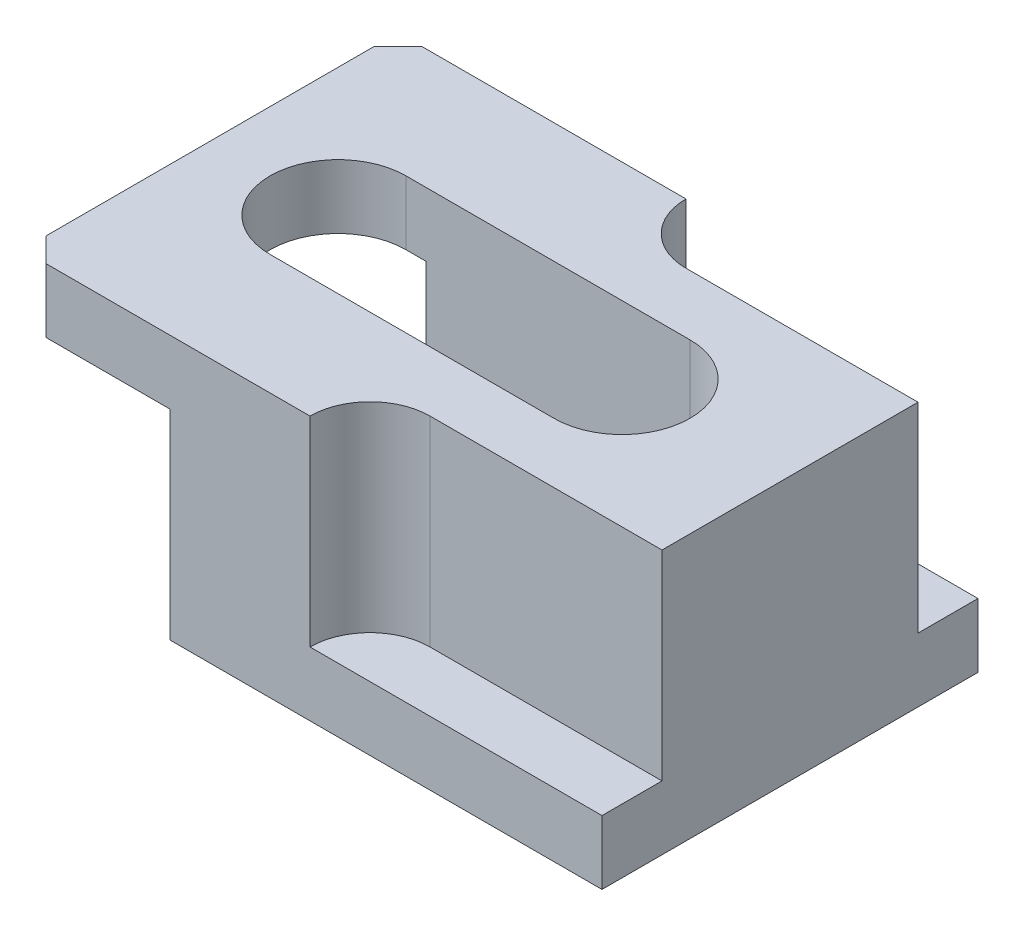
ISO-10303-21;
HEADER;
FILE_DESCRIPTION(('STEP AP214'),'2;1');
FILE_NAME('part.step','',(''),(''),'','','');
FILE_SCHEMA(('AUTOMOTIVE_DESIGN { 1 0 10303 214 1 1 1 1 }'));
ENDSEC;
DATA;
#1=APPLICATION_CONTEXT('core data for automotive mechanical design processes');
#2=APPLICATION_PROTOCOL_DEFINITION('international standard','automotive_design',2000,#1);
#3=PRODUCT_CONTEXT('',#1,'mechanical');
#4=PRODUCT('Part','Part','',(#3));
#5=PRODUCT_RELATED_PRODUCT_CATEGORY('part','',(#4));
#6=PRODUCT_DEFINITION_FORMATION('','',#4);
#7=PRODUCT_DEFINITION_CONTEXT('part definition',#1,'design');
#8=PRODUCT_DEFINITION('design','',#6,#7);
#9=PRODUCT_DEFINITION_SHAPE('','',#8);
#10=(LENGTH_UNIT() NAMED_UNIT(*) SI_UNIT(.MILLI.,.METRE.));
#11=(NAMED_UNIT(*) PLANE_ANGLE_UNIT() SI_UNIT($,.RADIAN.));
#12=(NAMED_UNIT(*) SI_UNIT($,.STERADIAN.) SOLID_ANGLE_UNIT());
#13=UNCERTAINTY_MEASURE_WITH_UNIT(LENGTH_MEASURE(1.E-05),#10,'distance_accuracy_value','');
#14=(GEOMETRIC_REPRESENTATION_CONTEXT(3) GLOBAL_UNCERTAINTY_ASSIGNED_CONTEXT((#13)) GLOBAL_UNIT_ASSIGNED_CONTEXT((#10,
#11,#12)) REPRESENTATION_CONTEXT('',''));
#15=CARTESIAN_POINT('',(0.,0.,0.));
#16=DIRECTION('',(0.,0.,1.));
#17=DIRECTION('',(1.,0.,0.));
#18=AXIS2_PLACEMENT_3D('',#15,#16,#17);
#19=CARTESIAN_POINT('',(0.,25.,-47.));
#20=DIRECTION('',(-1.,0.,0.));
#21=DIRECTION('',(0.,-1.,0.));
#22=AXIS2_PLACEMENT_3D('',#19,#20,#21);
#23=PLANE('',#22);
#24=DIRECTION('',(0.,-1.,0.));
#25=VECTOR('',#24,1.);
#26=CARTESIAN_POINT('',(0.,25.,-32.));
#27=LINE('',#26,#25);
#28=CARTESIAN_POINT('',(0.,25.,-32.));
#29=VERTEX_POINT('',#28);
#30=CARTESIAN_POINT('',(0.,8.,-32.));
#31=VERTEX_POINT('',#30);
#32=EDGE_CURVE('E237',#29,#31,#27,.T.);
#33=ORIENTED_EDGE('',*,*,#32,.F.);
#34=DIRECTION('',(0.,0.,1.));
#35=VECTOR('',#34,1.);
#36=CARTESIAN_POINT('',(0.,25.,-47.));
#37=LINE('',#36,#35);
#38=CARTESIAN_POINT('',(0.,25.,-47.));
#39=VERTEX_POINT('',#38);
#40=EDGE_CURVE('E315',#39,#29,#37,.T.);
#41=ORIENTED_EDGE('',*,*,#40,.F.);
#42=DIRECTION('',(0.,-1.,0.));
#43=VECTOR('',#42,1.);
#44=CARTESIAN_POINT('',(0.,25.,-47.));
#45=LINE('',#44,#43);
#46=CARTESIAN_POINT('',(0.,0.,-47.));
#47=VERTEX_POINT('',#46);
#48=EDGE_CURVE('E289',#39,#47,#45,.T.);
#49=ORIENTED_EDGE('',*,*,#48,.T.);
#50=DIRECTION('',(0.,0.,1.));
#51=VECTOR('',#50,1.);
#52=CARTESIAN_POINT('',(0.,0.,-47.));
#53=LINE('',#52,#51);
#54=CARTESIAN_POINT('',(0.,0.,0.));
#55=VERTEX_POINT('',#54);
#56=EDGE_CURVE('E300',#47,#55,#53,.T.);
#57=ORIENTED_EDGE('',*,*,#56,.T.);
#58=DIRECTION('',(0.,-1.,0.));
#59=VECTOR('',#58,1.);
#60=CARTESIAN_POINT('',(0.,25.,0.));
#61=LINE('',#60,#59);
#62=CARTESIAN_POINT('',(0.,25.,0.));
#63=VERTEX_POINT('',#62);
#64=EDGE_CURVE('E281',#63,#55,#61,.T.);
#65=ORIENTED_EDGE('',*,*,#64,.F.);
#66=CARTESIAN_POINT('',(0.,25.,-15.));
#67=VERTEX_POINT('',#66);
#68=EDGE_CURVE('E312',#67,#63,#37,.T.);
#69=ORIENTED_EDGE('',*,*,#68,.F.);
#70=DIRECTION('',(0.,1.,0.));
#71=VECTOR('',#70,1.);
#72=CARTESIAN_POINT('',(0.,25.,-15.));
#73=LINE('',#72,#71);
#74=CARTESIAN_POINT('',(0.,8.,-15.));
#75=VERTEX_POINT('',#74);
#76=EDGE_CURVE('E231',#75,#67,#73,.T.);
#77=ORIENTED_EDGE('',*,*,#76,.F.);
#78=DIRECTION('',(0.,0.,-1.));
#79=VECTOR('',#78,1.);
#80=CARTESIAN_POINT('',(0.,8.,-47.));
#81=LINE('',#80,#79);
#82=EDGE_CURVE('E197',#75,#31,#81,.T.);
#83=ORIENTED_EDGE('',*,*,#82,.T.);
#84=EDGE_LOOP('',(#33,#41,#49,#57,#65,#69,#77,#83));
#85=FACE_BOUND('',#84,.T.);
#86=ADVANCED_FACE('F50',(#85),#23,.T.);
#87=CARTESIAN_POINT('',(-18.5,25.,-47.));
#88=DIRECTION('',(0.,-1.,0.));
#89=DIRECTION('',(0.,0.,-1.));
#90=AXIS2_PLACEMENT_3D('',#87,#88,#89);
#91=PLANE('',#90);
#92=DIRECTION('',(0.,0.,1.));
#93=VECTOR('',#92,1.);
#94=CARTESIAN_POINT('',(-18.5,25.,-47.));
#95=LINE('',#94,#93);
#96=CARTESIAN_POINT('',(-18.5,25.,-44.));
#97=VERTEX_POINT('',#96);
#98=CARTESIAN_POINT('',(-18.5,25.,-3.));
#99=VERTEX_POINT('',#98);
#100=EDGE_CURVE('E316',#97,#99,#95,.T.);
#101=ORIENTED_EDGE('',*,*,#100,.F.);
#102=DIRECTION('',(0.707106781186549,0.,-0.707106781186546));
#103=VECTOR('',#102,1.);
#104=CARTESIAN_POINT('',(-17.,25.,-45.5));
#105=LINE('',#104,#103);
#106=CARTESIAN_POINT('',(-15.5,25.,-47.));
#107=VERTEX_POINT('',#106);
#108=EDGE_CURVE('E333',#97,#107,#105,.T.);
#109=ORIENTED_EDGE('',*,*,#108,.T.);
#110=DIRECTION('',(1.,0.,0.));
#111=VECTOR('',#110,1.);
#112=CARTESIAN_POINT('',(-18.5,25.,-47.));
#113=LINE('',#112,#111);
#114=EDGE_CURVE('E299',#107,#39,#113,.T.);
#115=ORIENTED_EDGE('',*,*,#114,.T.);
#116=ORIENTED_EDGE('',*,*,#40,.T.);
#117=DIRECTION('',(1.,0.,0.));
#118=VECTOR('',#117,1.);
#119=CARTESIAN_POINT('',(-18.5,25.,-32.));
#120=LINE('',#119,#118);
#121=CARTESIAN_POINT('',(-2.5,25.,-32.));
#122=VERTEX_POINT('',#121);
#123=EDGE_CURVE('E233',#122,#29,#120,.T.);
#124=ORIENTED_EDGE('',*,*,#123,.F.);
#125=CARTESIAN_POINT('',(-2.5,25.,-23.5));
#126=DIRECTION('',(0.,-1.,0.));
#127=DIRECTION('',(0.,0.,-1.));
#128=AXIS2_PLACEMENT_3D('',#125,#126,#127);
#129=CIRCLE('',#128,8.5);
#130=CARTESIAN_POINT('',(-2.5,25.,-15.));
#131=VERTEX_POINT('',#130);
#132=EDGE_CURVE('E236',#131,#122,#129,.T.);
#133=ORIENTED_EDGE('',*,*,#132,.F.);
#134=DIRECTION('',(-1.,0.,0.));
#135=VECTOR('',#134,1.);
#136=CARTESIAN_POINT('',(-18.5,25.,-15.));
#137=LINE('',#136,#135);
#138=EDGE_CURVE('E229',#67,#131,#137,.T.);
#139=ORIENTED_EDGE('',*,*,#138,.F.);
#140=ORIENTED_EDGE('',*,*,#68,.T.);
#141=DIRECTION('',(1.,0.,0.));
#142=VECTOR('',#141,1.);
#143=CARTESIAN_POINT('',(-18.5,25.,0.));
#144=LINE('',#143,#142);
#145=CARTESIAN_POINT('',(-15.5,25.,0.));
#146=VERTEX_POINT('',#145);
#147=EDGE_CURVE('E287',#146,#63,#144,.T.);
#148=ORIENTED_EDGE('',*,*,#147,.F.);
#149=DIRECTION('',(0.707106781186548,0.,0.707106781186548));
#150=VECTOR('',#149,1.);
#151=CARTESIAN_POINT('',(-40.5,25.,-25.));
#152=LINE('',#151,#150);
#153=EDGE_CURVE('E334',#146,#99,#152,.F.);
#154=ORIENTED_EDGE('',*,*,#153,.T.);
#155=EDGE_LOOP('',(#101,#109,#115,#116,#124,#133,#139,#140,#148,#154));
#156=FACE_BOUND('',#155,.T.);
#157=ADVANCED_FACE('F348',(#156),#91,.T.);
#158=CARTESIAN_POINT('',(-18.5,33.,-47.));
#159=DIRECTION('',(-1.,0.,0.));
#160=DIRECTION('',(0.,0.,1.));
#161=AXIS2_PLACEMENT_3D('',#158,#159,#160);
#162=PLANE('',#161);
#163=DIRECTION('',(0.,0.,1.));
#164=VECTOR('',#163,1.);
#165=CARTESIAN_POINT('',(-18.5,33.,-47.));
#166=LINE('',#165,#164);
#167=CARTESIAN_POINT('',(-18.5,33.,-44.));
#168=VERTEX_POINT('',#167);
#169=CARTESIAN_POINT('',(-18.5,33.,-3.));
#170=VERTEX_POINT('',#169);
#171=EDGE_CURVE('E317',#168,#170,#166,.T.);
#172=ORIENTED_EDGE('',*,*,#171,.F.);
#173=DIRECTION('',(0.,-1.,0.));
#174=VECTOR('',#173,1.);
#175=CARTESIAN_POINT('',(-18.5,25.,-44.));
#176=LINE('',#175,#174);
#177=EDGE_CURVE('E329',#168,#97,#176,.T.);
#178=ORIENTED_EDGE('',*,*,#177,.T.);
#179=ORIENTED_EDGE('',*,*,#100,.T.);
#180=DIRECTION('',(0.,1.,0.));
#181=VECTOR('',#180,1.);
#182=CARTESIAN_POINT('',(-18.5,33.,-3.));
#183=LINE('',#182,#181);
#184=EDGE_CURVE('E327',#99,#170,#183,.T.);
#185=ORIENTED_EDGE('',*,*,#184,.T.);
#186=EDGE_LOOP('',(#172,#178,#179,#185));
#187=FACE_BOUND('',#186,.T.);
#188=ADVANCED_FACE('F342',(#187),#162,.T.);
#189=CARTESIAN_POINT('',(54.,33.,-47.));
#190=DIRECTION('',(0.,1.,0.));
#191=DIRECTION('',(0.,0.,1.));
#192=AXIS2_PLACEMENT_3D('',#189,#190,#191);
#193=PLANE('',#192);
#194=CARTESIAN_POINT('',(-2.5,33.,-23.5));
#195=DIRECTION('',(0.,1.,0.));
#196=DIRECTION('',(0.,0.,1.));
#197=AXIS2_PLACEMENT_3D('',#194,#195,#196);
#198=CIRCLE('',#197,8.5);
#199=CARTESIAN_POINT('',(-2.5,33.,-32.));
#200=VERTEX_POINT('',#199);
#201=CARTESIAN_POINT('',(-2.5,33.,-15.));
#202=VERTEX_POINT('',#201);
#203=EDGE_CURVE('E218',#200,#202,#198,.T.);
#204=ORIENTED_EDGE('',*,*,#203,.F.);
#205=DIRECTION('',(-1.,0.,0.));
#206=VECTOR('',#205,1.);
#207=CARTESIAN_POINT('',(-2.5,33.,-32.));
#208=LINE('',#207,#206);
#209=CARTESIAN_POINT('',(33.,33.,-32.));
#210=VERTEX_POINT('',#209);
#211=EDGE_CURVE('E199',#210,#200,#208,.T.);
#212=ORIENTED_EDGE('',*,*,#211,.F.);
#213=CARTESIAN_POINT('',(33.,33.,-23.5));
#214=DIRECTION('',(0.,1.,0.));
#215=DIRECTION('',(0.,0.,1.));
#216=AXIS2_PLACEMENT_3D('',#213,#214,#215);
#217=CIRCLE('',#216,8.5);
#218=CARTESIAN_POINT('',(33.,33.,-15.));
#219=VERTEX_POINT('',#218);
#220=EDGE_CURVE('E225',#219,#210,#217,.T.);
#221=ORIENTED_EDGE('',*,*,#220,.F.);
#222=DIRECTION('',(1.,0.,0.));
#223=VECTOR('',#222,1.);
#224=CARTESIAN_POINT('',(-2.5,33.,-15.));
#225=LINE('',#224,#223);
#226=EDGE_CURVE('E210',#202,#219,#225,.T.);
#227=ORIENTED_EDGE('',*,*,#226,.F.);
#228=EDGE_LOOP('',(#204,#212,#221,#227));
#229=FACE_BOUND('',#228,.T.);
#230=DIRECTION('',(-1.,0.,0.));
#231=VECTOR('',#230,1.);
#232=CARTESIAN_POINT('',(54.,33.,-47.));
#233=LINE('',#232,#231);
#234=CARTESIAN_POINT('',(17.5,33.,-47.));
#235=VERTEX_POINT('',#234);
#236=CARTESIAN_POINT('',(-15.5,33.,-47.));
#237=VERTEX_POINT('',#236);
#238=EDGE_CURVE('E296',#235,#237,#233,.T.);
#239=ORIENTED_EDGE('',*,*,#238,.T.);
#240=DIRECTION('',(-0.707106781186549,0.,0.707106781186546));
#241=VECTOR('',#240,1.);
#242=CARTESIAN_POINT('',(19.2500000000002,33.,-81.75));
#243=LINE('',#242,#241);
#244=EDGE_CURVE('E57',#237,#168,#243,.T.);
#245=ORIENTED_EDGE('',*,*,#244,.T.);
#246=ORIENTED_EDGE('',*,*,#171,.T.);
#247=DIRECTION('',(-0.707106781186548,0.,-0.707106781186548));
#248=VECTOR('',#247,1.);
#249=CARTESIAN_POINT('',(-4.25,33.,11.25));
#250=LINE('',#249,#248);
#251=CARTESIAN_POINT('',(-15.5,33.,0.));
#252=VERTEX_POINT('',#251);
#253=EDGE_CURVE('E64',#170,#252,#250,.F.);
#254=ORIENTED_EDGE('',*,*,#253,.T.);
#255=DIRECTION('',(-1.,0.,0.));
#256=VECTOR('',#255,1.);
#257=CARTESIAN_POINT('',(54.,33.,0.));
#258=LINE('',#257,#256);
#259=CARTESIAN_POINT('',(17.5,33.,0.));
#260=VERTEX_POINT('',#259);
#261=EDGE_CURVE('E310',#260,#252,#258,.T.);
#262=ORIENTED_EDGE('',*,*,#261,.F.);
#263=CARTESIAN_POINT('',(25.,33.,0.));
#264=DIRECTION('',(0.,1.,0.));
#265=DIRECTION('',(0.,0.,1.));
#266=AXIS2_PLACEMENT_3D('',#263,#264,#265);
#267=CIRCLE('',#266,7.5);
#268=CARTESIAN_POINT('',(25.,33.,-7.5));
#269=VERTEX_POINT('',#268);
#270=EDGE_CURVE('E266',#269,#260,#267,.T.);
#271=ORIENTED_EDGE('',*,*,#270,.F.);
#272=DIRECTION('',(-1.,0.,0.));
#273=VECTOR('',#272,1.);
#274=CARTESIAN_POINT('',(54.,33.,-7.5));
#275=LINE('',#274,#273);
#276=CARTESIAN_POINT('',(54.,33.,-7.5));
#277=VERTEX_POINT('',#276);
#278=EDGE_CURVE('E259',#277,#269,#275,.T.);
#279=ORIENTED_EDGE('',*,*,#278,.F.);
#280=DIRECTION('',(0.,0.,1.));
#281=VECTOR('',#280,1.);
#282=CARTESIAN_POINT('',(54.,33.,-47.));
#283=LINE('',#282,#281);
#284=CARTESIAN_POINT('',(54.,33.,-39.5));
#285=VERTEX_POINT('',#284);
#286=EDGE_CURVE('E321',#285,#277,#283,.T.);
#287=ORIENTED_EDGE('',*,*,#286,.F.);
#288=DIRECTION('',(1.,0.,0.));
#289=VECTOR('',#288,1.);
#290=CARTESIAN_POINT('',(54.,33.,-39.5));
#291=LINE('',#290,#289);
#292=CARTESIAN_POINT('',(25.,33.,-39.5));
#293=VERTEX_POINT('',#292);
#294=EDGE_CURVE('E243',#293,#285,#291,.T.);
#295=ORIENTED_EDGE('',*,*,#294,.F.);
#296=CARTESIAN_POINT('',(25.,33.,-47.));
#297=DIRECTION('',(0.,1.,0.));
#298=DIRECTION('',(0.,0.,1.));
#299=AXIS2_PLACEMENT_3D('',#296,#297,#298);
#300=CIRCLE('',#299,7.5);
#301=EDGE_CURVE('E238',#235,#293,#300,.T.);
#302=ORIENTED_EDGE('',*,*,#301,.F.);
#303=EDGE_LOOP('',(#239,#245,#246,#254,#262,#271,#279,#287,#295,#302));
#304=FACE_BOUND('',#303,.T.);
#305=ADVANCED_FACE('F340',(#229,#304),#193,.T.);
#306=CARTESIAN_POINT('',(54.,8.,-47.));
#307=DIRECTION('',(1.,0.,0.));
#308=DIRECTION('',(0.,0.,-1.));
#309=AXIS2_PLACEMENT_3D('',#306,#307,#308);
#310=PLANE('',#309);
#311=DIRECTION('',(0.,1.,0.));
#312=VECTOR('',#311,1.);
#313=CARTESIAN_POINT('',(54.,8.,-39.5));
#314=LINE('',#313,#312);
#315=CARTESIAN_POINT('',(54.,8.,-39.5));
#316=VERTEX_POINT('',#315);
#317=EDGE_CURVE('E258',#316,#285,#314,.T.);
#318=ORIENTED_EDGE('',*,*,#317,.T.);
#319=ORIENTED_EDGE('',*,*,#286,.T.);
#320=DIRECTION('',(0.,1.,0.));
#321=VECTOR('',#320,1.);
#322=CARTESIAN_POINT('',(54.,8.,-7.5));
#323=LINE('',#322,#321);
#324=CARTESIAN_POINT('',(54.,8.,-7.5));
#325=VERTEX_POINT('',#324);
#326=EDGE_CURVE('E273',#325,#277,#323,.T.);
#327=ORIENTED_EDGE('',*,*,#326,.F.);
#328=DIRECTION('',(0.,0.,-1.));
#329=VECTOR('',#328,1.);
#330=CARTESIAN_POINT('',(54.,8.,0.));
#331=LINE('',#330,#329);
#332=CARTESIAN_POINT('',(54.,8.,0.));
#333=VERTEX_POINT('',#332);
#334=EDGE_CURVE('E264',#333,#325,#331,.T.);
#335=ORIENTED_EDGE('',*,*,#334,.F.);
#336=DIRECTION('',(0.,1.,0.));
#337=VECTOR('',#336,1.);
#338=CARTESIAN_POINT('',(54.,8.,0.));
#339=LINE('',#338,#337);
#340=CARTESIAN_POINT('',(54.,0.,0.));
#341=VERTEX_POINT('',#340);
#342=EDGE_CURVE('E308',#341,#333,#339,.T.);
#343=ORIENTED_EDGE('',*,*,#342,.F.);
#344=DIRECTION('',(0.,0.,1.));
#345=VECTOR('',#344,1.);
#346=CARTESIAN_POINT('',(54.,0.,-47.));
#347=LINE('',#346,#345);
#348=CARTESIAN_POINT('',(54.,0.,-47.));
#349=VERTEX_POINT('',#348);
#350=EDGE_CURVE('E323',#349,#341,#347,.T.);
#351=ORIENTED_EDGE('',*,*,#350,.F.);
#352=DIRECTION('',(0.,1.,0.));
#353=VECTOR('',#352,1.);
#354=CARTESIAN_POINT('',(54.,0.,-47.));
#355=LINE('',#354,#353);
#356=CARTESIAN_POINT('',(54.,8.,-47.));
#357=VERTEX_POINT('',#356);
#358=EDGE_CURVE('E291',#349,#357,#355,.T.);
#359=ORIENTED_EDGE('',*,*,#358,.T.);
#360=DIRECTION('',(0.,0.,-1.));
#361=VECTOR('',#360,1.);
#362=CARTESIAN_POINT('',(54.,8.,-47.));
#363=LINE('',#362,#361);
#364=EDGE_CURVE('E247',#316,#357,#363,.T.);
#365=ORIENTED_EDGE('',*,*,#364,.F.);
#366=EDGE_LOOP('',(#318,#319,#327,#335,#343,#351,#359,#365));
#367=FACE_BOUND('',#366,.T.);
#368=ADVANCED_FACE('F373',(#367),#310,.T.);
#369=CARTESIAN_POINT('',(0.,0.,-47.));
#370=DIRECTION('',(0.,-1.,0.));
#371=DIRECTION('',(0.,0.,-1.));
#372=AXIS2_PLACEMENT_3D('',#369,#370,#371);
#373=PLANE('',#372);
#374=DIRECTION('',(1.,0.,0.));
#375=VECTOR('',#374,1.);
#376=CARTESIAN_POINT('',(0.,0.,0.));
#377=LINE('',#376,#375);
#378=EDGE_CURVE('E305',#55,#341,#377,.T.);
#379=ORIENTED_EDGE('',*,*,#378,.F.);
#380=ORIENTED_EDGE('',*,*,#56,.F.);
#381=DIRECTION('',(1.,0.,0.));
#382=VECTOR('',#381,1.);
#383=CARTESIAN_POINT('',(0.,0.,-47.));
#384=LINE('',#383,#382);
#385=EDGE_CURVE('E288',#47,#349,#384,.T.);
#386=ORIENTED_EDGE('',*,*,#385,.T.);
#387=ORIENTED_EDGE('',*,*,#350,.T.);
#388=EDGE_LOOP('',(#379,#380,#386,#387));
#389=FACE_BOUND('',#388,.T.);
#390=ADVANCED_FACE('F379',(#389),#373,.T.);
#391=CARTESIAN_POINT('',(0.,0.,-47.));
#392=DIRECTION('',(0.,0.,1.));
#393=DIRECTION('',(1.,0.,0.));
#394=AXIS2_PLACEMENT_3D('',#391,#392,#393);
#395=PLANE('',#394);
#396=ORIENTED_EDGE('',*,*,#114,.F.);
#397=DIRECTION('',(0.,1.,0.));
#398=VECTOR('',#397,1.);
#399=CARTESIAN_POINT('',(-15.5,33.,-47.));
#400=LINE('',#399,#398);
#401=EDGE_CURVE('E72',#107,#237,#400,.T.);
#402=ORIENTED_EDGE('',*,*,#401,.T.);
#403=ORIENTED_EDGE('',*,*,#238,.F.);
#404=DIRECTION('',(0.,1.,0.));
#405=VECTOR('',#404,1.);
#406=CARTESIAN_POINT('',(17.5,8.,-47.));
#407=LINE('',#406,#405);
#408=CARTESIAN_POINT('',(17.5,8.,-47.));
#409=VERTEX_POINT('',#408);
#410=EDGE_CURVE('E252',#409,#235,#407,.T.);
#411=ORIENTED_EDGE('',*,*,#410,.F.);
#412=DIRECTION('',(-1.,0.,0.));
#413=VECTOR('',#412,1.);
#414=CARTESIAN_POINT('',(25.,8.,-47.));
#415=LINE('',#414,#413);
#416=EDGE_CURVE('E241',#357,#409,#415,.T.);
#417=ORIENTED_EDGE('',*,*,#416,.F.);
#418=ORIENTED_EDGE('',*,*,#358,.F.);
#419=ORIENTED_EDGE('',*,*,#385,.F.);
#420=ORIENTED_EDGE('',*,*,#48,.F.);
#421=EDGE_LOOP('',(#396,#402,#403,#411,#417,#418,#419,#420));
#422=FACE_BOUND('',#421,.T.);
#423=ADVANCED_FACE('F354',(#422),#395,.F.);
#424=CARTESIAN_POINT('',(0.,0.,0.));
#425=DIRECTION('',(0.,0.,1.));
#426=DIRECTION('',(1.,0.,0.));
#427=AXIS2_PLACEMENT_3D('',#424,#425,#426);
#428=PLANE('',#427);
#429=ORIENTED_EDGE('',*,*,#261,.T.);
#430=DIRECTION('',(0.,-1.,0.));
#431=VECTOR('',#430,1.);
#432=CARTESIAN_POINT('',(-15.5,0.,0.));
#433=LINE('',#432,#431);
#434=EDGE_CURVE('E11',#252,#146,#433,.T.);
#435=ORIENTED_EDGE('',*,*,#434,.T.);
#436=ORIENTED_EDGE('',*,*,#147,.T.);
#437=ORIENTED_EDGE('',*,*,#64,.T.);
#438=ORIENTED_EDGE('',*,*,#378,.T.);
#439=ORIENTED_EDGE('',*,*,#342,.T.);
#440=DIRECTION('',(1.,0.,0.));
#441=VECTOR('',#440,1.);
#442=CARTESIAN_POINT('',(25.,8.,0.));
#443=LINE('',#442,#441);
#444=CARTESIAN_POINT('',(17.5,8.,0.));
#445=VERTEX_POINT('',#444);
#446=EDGE_CURVE('E263',#445,#333,#443,.T.);
#447=ORIENTED_EDGE('',*,*,#446,.F.);
#448=DIRECTION('',(0.,1.,0.));
#449=VECTOR('',#448,1.);
#450=CARTESIAN_POINT('',(17.5,8.,0.));
#451=LINE('',#450,#449);
#452=EDGE_CURVE('E279',#445,#260,#451,.T.);
#453=ORIENTED_EDGE('',*,*,#452,.T.);
#454=EDGE_LOOP('',(#429,#435,#436,#437,#438,#439,#447,#453));
#455=FACE_BOUND('',#454,.T.);
#456=ADVANCED_FACE('F432',(#455),#428,.T.);
#457=CARTESIAN_POINT('',(25.,8.,0.));
#458=DIRECTION('',(0.,1.,0.));
#459=DIRECTION('',(0.,0.,1.));
#460=AXIS2_PLACEMENT_3D('',#457,#458,#459);
#461=CYLINDRICAL_SURFACE('',#460,7.5);
#462=ORIENTED_EDGE('',*,*,#270,.T.);
#463=ORIENTED_EDGE('',*,*,#452,.F.);
#464=CARTESIAN_POINT('',(25.,8.,0.));
#465=DIRECTION('',(0.,1.,0.));
#466=DIRECTION('',(0.,0.,1.));
#467=AXIS2_PLACEMENT_3D('',#464,#465,#466);
#468=CIRCLE('',#467,7.5);
#469=CARTESIAN_POINT('',(25.,8.,-7.5));
#470=VERTEX_POINT('',#469);
#471=EDGE_CURVE('E275',#470,#445,#468,.T.);
#472=ORIENTED_EDGE('',*,*,#471,.F.);
#473=DIRECTION('',(0.,1.,0.));
#474=VECTOR('',#473,1.);
#475=CARTESIAN_POINT('',(25.,8.,-7.5));
#476=LINE('',#475,#474);
#477=EDGE_CURVE('E282',#470,#269,#476,.T.);
#478=ORIENTED_EDGE('',*,*,#477,.T.);
#479=EDGE_LOOP('',(#462,#463,#472,#478));
#480=FACE_BOUND('',#479,.T.);
#481=ADVANCED_FACE('F431',(#480),#461,.F.);
#482=CARTESIAN_POINT('',(54.,8.,-7.5));
#483=DIRECTION('',(0.,0.,-1.));
#484=DIRECTION('',(-1.,0.,0.));
#485=AXIS2_PLACEMENT_3D('',#482,#483,#484);
#486=PLANE('',#485);
#487=ORIENTED_EDGE('',*,*,#278,.T.);
#488=ORIENTED_EDGE('',*,*,#477,.F.);
#489=DIRECTION('',(-1.,0.,0.));
#490=VECTOR('',#489,1.);
#491=CARTESIAN_POINT('',(54.,8.,-7.5));
#492=LINE('',#491,#490);
#493=EDGE_CURVE('E267',#325,#470,#492,.T.);
#494=ORIENTED_EDGE('',*,*,#493,.F.);
#495=ORIENTED_EDGE('',*,*,#326,.T.);
#496=EDGE_LOOP('',(#487,#488,#494,#495));
#497=FACE_BOUND('',#496,.T.);
#498=ADVANCED_FACE('F427',(#497),#486,.F.);
#499=CARTESIAN_POINT('',(25.,8.,0.));
#500=DIRECTION('',(0.,1.,0.));
#501=DIRECTION('',(0.,0.,1.));
#502=AXIS2_PLACEMENT_3D('',#499,#500,#501);
#503=PLANE('',#502);
#504=ORIENTED_EDGE('',*,*,#446,.T.);
#505=ORIENTED_EDGE('',*,*,#334,.T.);
#506=ORIENTED_EDGE('',*,*,#493,.T.);
#507=ORIENTED_EDGE('',*,*,#471,.T.);
#508=EDGE_LOOP('',(#504,#505,#506,#507));
#509=FACE_BOUND('',#508,.T.);
#510=ADVANCED_FACE('F425',(#509),#503,.T.);
#511=CARTESIAN_POINT('',(54.,8.,-39.5));
#512=DIRECTION('',(0.,0.,1.));
#513=DIRECTION('',(1.,0.,0.));
#514=AXIS2_PLACEMENT_3D('',#511,#512,#513);
#515=PLANE('',#514);
#516=ORIENTED_EDGE('',*,*,#294,.T.);
#517=ORIENTED_EDGE('',*,*,#317,.F.);
#518=DIRECTION('',(1.,0.,0.));
#519=VECTOR('',#518,1.);
#520=CARTESIAN_POINT('',(54.,8.,-39.5));
#521=LINE('',#520,#519);
#522=CARTESIAN_POINT('',(25.,8.,-39.5));
#523=VERTEX_POINT('',#522);
#524=EDGE_CURVE('E246',#523,#316,#521,.T.);
#525=ORIENTED_EDGE('',*,*,#524,.F.);
#526=DIRECTION('',(0.,1.,0.));
#527=VECTOR('',#526,1.);
#528=CARTESIAN_POINT('',(25.,8.,-39.5));
#529=LINE('',#528,#527);
#530=EDGE_CURVE('E257',#523,#293,#529,.T.);
#531=ORIENTED_EDGE('',*,*,#530,.T.);
#532=EDGE_LOOP('',(#516,#517,#525,#531));
#533=FACE_BOUND('',#532,.T.);
#534=ADVANCED_FACE('F420',(#533),#515,.F.);
#535=CARTESIAN_POINT('',(25.,8.,-47.));
#536=DIRECTION('',(0.,1.,0.));
#537=DIRECTION('',(0.,0.,1.));
#538=AXIS2_PLACEMENT_3D('',#535,#536,#537);
#539=CYLINDRICAL_SURFACE('',#538,7.5);
#540=ORIENTED_EDGE('',*,*,#301,.T.);
#541=ORIENTED_EDGE('',*,*,#530,.F.);
#542=CARTESIAN_POINT('',(25.,8.,-47.));
#543=DIRECTION('',(0.,1.,0.));
#544=DIRECTION('',(0.,0.,1.));
#545=AXIS2_PLACEMENT_3D('',#542,#543,#544);
#546=CIRCLE('',#545,7.5);
#547=EDGE_CURVE('E244',#409,#523,#546,.T.);
#548=ORIENTED_EDGE('',*,*,#547,.F.);
#549=ORIENTED_EDGE('',*,*,#410,.T.);
#550=EDGE_LOOP('',(#540,#541,#548,#549));
#551=FACE_BOUND('',#550,.T.);
#552=ADVANCED_FACE('F417',(#551),#539,.F.);
#553=CARTESIAN_POINT('',(25.,8.,-47.));
#554=DIRECTION('',(0.,1.,0.));
#555=DIRECTION('',(0.,0.,1.));
#556=AXIS2_PLACEMENT_3D('',#553,#554,#555);
#557=PLANE('',#556);
#558=ORIENTED_EDGE('',*,*,#416,.T.);
#559=ORIENTED_EDGE('',*,*,#547,.T.);
#560=ORIENTED_EDGE('',*,*,#524,.T.);
#561=ORIENTED_EDGE('',*,*,#364,.T.);
#562=EDGE_LOOP('',(#558,#559,#560,#561));
#563=FACE_BOUND('',#562,.T.);
#564=ADVANCED_FACE('F412',(#563),#557,.T.);
#565=CARTESIAN_POINT('',(-2.5,8.,-23.5));
#566=DIRECTION('',(0.,1.,0.));
#567=DIRECTION('',(0.,0.,1.));
#568=AXIS2_PLACEMENT_3D('',#565,#566,#567);
#569=CYLINDRICAL_SURFACE('',#568,8.5);
#570=ORIENTED_EDGE('',*,*,#132,.T.);
#571=DIRECTION('',(0.,1.,0.));
#572=VECTOR('',#571,1.);
#573=CARTESIAN_POINT('',(-2.5,8.,-32.));
#574=LINE('',#573,#572);
#575=EDGE_CURVE('E226',#122,#200,#574,.T.);
#576=ORIENTED_EDGE('',*,*,#575,.T.);
#577=ORIENTED_EDGE('',*,*,#203,.T.);
#578=DIRECTION('',(0.,1.,0.));
#579=VECTOR('',#578,1.);
#580=CARTESIAN_POINT('',(-2.5,8.,-15.));
#581=LINE('',#580,#579);
#582=EDGE_CURVE('E215',#131,#202,#581,.T.);
#583=ORIENTED_EDGE('',*,*,#582,.F.);
#584=EDGE_LOOP('',(#570,#576,#577,#583));
#585=FACE_BOUND('',#584,.T.);
#586=ADVANCED_FACE('F369',(#585),#569,.F.);
#587=CARTESIAN_POINT('',(-2.5,8.,-32.));
#588=DIRECTION('',(0.,0.,-1.));
#589=DIRECTION('',(-1.,0.,0.));
#590=AXIS2_PLACEMENT_3D('',#587,#588,#589);
#591=PLANE('',#590);
#592=ORIENTED_EDGE('',*,*,#32,.T.);
#593=DIRECTION('',(-1.,0.,0.));
#594=VECTOR('',#593,1.);
#595=CARTESIAN_POINT('',(-2.5,8.,-32.));
#596=LINE('',#595,#594);
#597=CARTESIAN_POINT('',(33.,8.,-32.));
#598=VERTEX_POINT('',#597);
#599=EDGE_CURVE('E214',#598,#31,#596,.T.);
#600=ORIENTED_EDGE('',*,*,#599,.F.);
#601=DIRECTION('',(0.,1.,0.));
#602=VECTOR('',#601,1.);
#603=CARTESIAN_POINT('',(33.,8.,-32.));
#604=LINE('',#603,#602);
#605=EDGE_CURVE('E211',#598,#210,#604,.T.);
#606=ORIENTED_EDGE('',*,*,#605,.T.);
#607=ORIENTED_EDGE('',*,*,#211,.T.);
#608=ORIENTED_EDGE('',*,*,#575,.F.);
#609=ORIENTED_EDGE('',*,*,#123,.T.);
#610=EDGE_LOOP('',(#592,#600,#606,#607,#608,#609));
#611=FACE_BOUND('',#610,.T.);
#612=ADVANCED_FACE('F364',(#611),#591,.F.);
#613=CARTESIAN_POINT('',(33.,8.,-23.5));
#614=DIRECTION('',(0.,1.,0.));
#615=DIRECTION('',(0.,0.,1.));
#616=AXIS2_PLACEMENT_3D('',#613,#614,#615);
#617=CYLINDRICAL_SURFACE('',#616,8.5);
#618=ORIENTED_EDGE('',*,*,#220,.T.);
#619=ORIENTED_EDGE('',*,*,#605,.F.);
#620=CARTESIAN_POINT('',(33.,8.,-23.5));
#621=DIRECTION('',(0.,1.,0.));
#622=DIRECTION('',(0.,0.,1.));
#623=AXIS2_PLACEMENT_3D('',#620,#621,#622);
#624=CIRCLE('',#623,8.5);
#625=CARTESIAN_POINT('',(33.,8.,-15.));
#626=VERTEX_POINT('',#625);
#627=EDGE_CURVE('E193',#626,#598,#624,.T.);
#628=ORIENTED_EDGE('',*,*,#627,.F.);
#629=DIRECTION('',(0.,1.,0.));
#630=VECTOR('',#629,1.);
#631=CARTESIAN_POINT('',(33.,8.,-15.));
#632=LINE('',#631,#630);
#633=EDGE_CURVE('E201',#626,#219,#632,.T.);
#634=ORIENTED_EDGE('',*,*,#633,.T.);
#635=EDGE_LOOP('',(#618,#619,#628,#634));
#636=FACE_BOUND('',#635,.T.);
#637=ADVANCED_FACE('F212',(#636),#617,.F.);
#638=CARTESIAN_POINT('',(-2.5,8.,-15.));
#639=DIRECTION('',(0.,0.,1.));
#640=DIRECTION('',(1.,0.,0.));
#641=AXIS2_PLACEMENT_3D('',#638,#639,#640);
#642=PLANE('',#641);
#643=ORIENTED_EDGE('',*,*,#76,.T.);
#644=ORIENTED_EDGE('',*,*,#138,.T.);
#645=ORIENTED_EDGE('',*,*,#582,.T.);
#646=ORIENTED_EDGE('',*,*,#226,.T.);
#647=ORIENTED_EDGE('',*,*,#633,.F.);
#648=DIRECTION('',(1.,0.,0.));
#649=VECTOR('',#648,1.);
#650=CARTESIAN_POINT('',(-2.5,8.,-15.));
#651=LINE('',#650,#649);
#652=EDGE_CURVE('E188',#75,#626,#651,.T.);
#653=ORIENTED_EDGE('',*,*,#652,.F.);
#654=EDGE_LOOP('',(#643,#644,#645,#646,#647,#653));
#655=FACE_BOUND('',#654,.T.);
#656=ADVANCED_FACE('F204',(#655),#642,.F.);
#657=CARTESIAN_POINT('',(-2.5,8.,-23.5));
#658=DIRECTION('',(0.,1.,0.));
#659=DIRECTION('',(0.,0.,1.));
#660=AXIS2_PLACEMENT_3D('',#657,#658,#659);
#661=PLANE('',#660);
#662=ORIENTED_EDGE('',*,*,#652,.T.);
#663=ORIENTED_EDGE('',*,*,#627,.T.);
#664=ORIENTED_EDGE('',*,*,#599,.T.);
#665=ORIENTED_EDGE('',*,*,#82,.F.);
#666=EDGE_LOOP('',(#662,#663,#664,#665));
#667=FACE_BOUND('',#666,.T.);
#668=ADVANCED_FACE('F194',(#667),#661,.T.);
#669=CARTESIAN_POINT('',(-18.5,33.,-44.));
#670=DIRECTION('',(-0.707106781186546,0.,-0.707106781186549));
#671=DIRECTION('',(0.,1.,0.));
#672=AXIS2_PLACEMENT_3D('',#669,#670,#671);
#673=PLANE('',#672);
#674=ORIENTED_EDGE('',*,*,#244,.F.);
#675=ORIENTED_EDGE('',*,*,#401,.F.);
#676=ORIENTED_EDGE('',*,*,#108,.F.);
#677=ORIENTED_EDGE('',*,*,#177,.F.);
#678=EDGE_LOOP('',(#674,#675,#676,#677));
#679=FACE_BOUND('',#678,.T.);
#680=ADVANCED_FACE('F346',(#679),#673,.T.);
#681=CARTESIAN_POINT('',(-15.5,0.,0.));
#682=DIRECTION('',(0.707106781186547,0.,-0.707106781186547));
#683=DIRECTION('',(0.,-1.,0.));
#684=AXIS2_PLACEMENT_3D('',#681,#682,#683);
#685=PLANE('',#684);
#686=ORIENTED_EDGE('',*,*,#253,.F.);
#687=ORIENTED_EDGE('',*,*,#184,.F.);
#688=ORIENTED_EDGE('',*,*,#153,.F.);
#689=ORIENTED_EDGE('',*,*,#434,.F.);
#690=EDGE_LOOP('',(#686,#687,#688,#689));
#691=FACE_BOUND('',#690,.T.);
#692=ADVANCED_FACE('F49',(#691),#685,.F.);
#693=CLOSED_SHELL('',(#86,#157,#188,#305,#368,#390,#423,#456,#481,#498,#510,#534,#552,#564,#586,
#612,#637,#656,#668,#680,#692));
#694=MANIFOLD_SOLID_BREP('B2',#693);
#695=ADVANCED_BREP_SHAPE_REPRESENTATION('',(#18,#694),#14);
#696=SHAPE_DEFINITION_REPRESENTATION(#9,#695);
ENDSEC;
END-ISO-10303-21;
